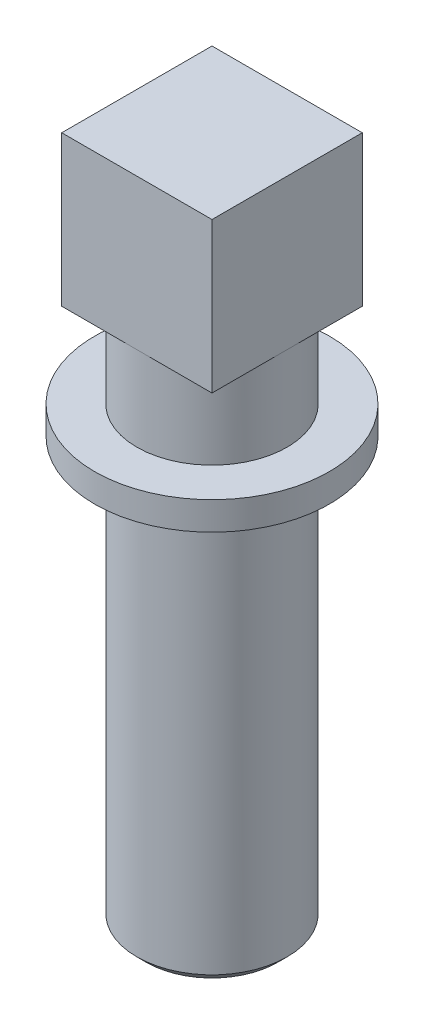
from build123d import *

# Parameters (mm, degrees)
SHANK_SKETCH_16_R          = 8
SHANK_16X45_DEPTH          = 45
SHANK_CHAMFER_1X45_SIZE    = 1
COLLAR_SKETCH_25_R         = 12.5
COLLAR_25X3_DEPTH          = 3
NECK_SKETCH_16_R           = 8
NECK_16X9_DEPTH            = 9
SQUARE_HEAD_SKETCH_16X16_W = 16
SQUARE_HEAD_SKETCH_16X16_H = 16
SQUARE_HEAD_16X16X16_DEPTH = 16


with BuildPart() as part:
    # Shank Sketch Ø16 → Shank Ø16x45 (new body)
    with BuildSketch(Plane(origin=(0, 0, 0), x_dir=(1, 0, 0), z_dir=(0, 1, 0))):
        with Locations(Location((0, 0, 0), (0, 0, 90))):
            Circle(SHANK_SKETCH_16_R)
    extrude(amount=SHANK_16X45_DEPTH)

    # Shank Chamfer 1x45°
    shank_chamfer_1x45_edges = [part.edges().sort_by_distance(p)[0] for p in [
        (0, 0, 8),
    ]]
    chamfer(shank_chamfer_1x45_edges, length=SHANK_CHAMFER_1X45_SIZE)

    # Collar Sketch Ø25 → Collar Ø25x3 (add)
    with BuildSketch(Plane(origin=(0, 45, 0), x_dir=(1, 0, 0), z_dir=(0, 1, 0))):
        with Locations(Location((0, 0, 0), (0, 0, 270))):
            Circle(COLLAR_SKETCH_25_R)
    extrude(amount=COLLAR_25X3_DEPTH)

    # Neck Sketch Ø16 → Neck Ø16x9 (add)
    with BuildSketch(Plane(origin=(0, 48, 0), x_dir=(1, 0, 0), z_dir=(0, 1, 0))):
        with Locations(Location((0, 0, 0), (0, 0, 90))):
            Circle(NECK_SKETCH_16_R)
    extrude(amount=NECK_16X9_DEPTH)

    # Square Head Sketch 16x16 → Square Head 16x16x16 (add)
    with BuildSketch(Plane(origin=(0, 57, 0), x_dir=(1, 0, 0), z_dir=(0, 1, 0))):
        Rectangle(SQUARE_HEAD_SKETCH_16X16_W, SQUARE_HEAD_SKETCH_16X16_H)
    extrude(amount=SQUARE_HEAD_16X16X16_DEPTH)


solid = part.part
